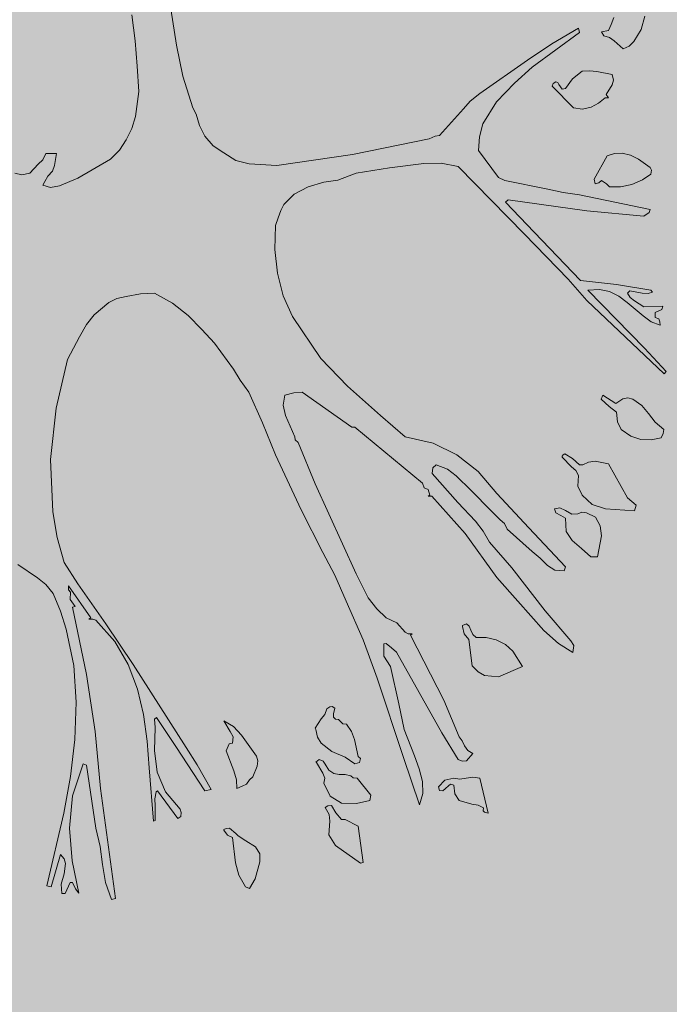
# Model space of a CAD drawing. Units: inches. Extents: x 84 to 1044, y -280 to 906.
# Tile 76 of 105: x 720.2 to 732.52, y 481.17 to 499.87. Entities that reach past the tile are written whole.
import ezdxf

# ---------------------------------------------------------------- set-up
doc = ezdxf.new("R2010")
doc.units = ezdxf.units.IN
doc.layers.add('A-ANNO-DIMS', color=2, linetype='Continuous', lineweight=18)
doc.layers.add('L-PLNT', color=114, linetype='Continuous', lineweight=15)
doc.layers.add('L-PLNT-PATT', color=9, linetype='Continuous', lineweight=9, true_color=0xafd9aa)
doc.styles.get("Standard").update_dxf_attribs({"font": 'arial.ttf'})
doc.dimstyles.get("Standard").update_dxf_attribs({"dimtxt": 0.18, "dimasz": 0.18, "dimexe": 0.18, "dimexo": 0.0625, "dimgap": 0.09, "dimtad": 0, "dimtih": 1, "dimtoh": 1, "dimdec": 4, "dimzin": 0, "dimdsep": 46, "dimtxsty": 'Standard', "dimcen": 0.09, "dimadec": 0, "dimazin": 0, "dimtfac": 1, "dimtdec": 4, "dimtofl": 0, "dimtmove": 0, "dimatfit": 3, "dimfxl": 1, "dimtolj": 1, "dimtzin": 0, "dimarcsym": 0})

# ---------------------------------------------------------------- blocks, each defined once
blk = doc.blocks.new('A$C37E508DF')
for p, q in [((0.7911, 1.1436), (0.8027, 1.0677)), ((0.7512, 1.0728), (0.7469, 1.1054)), ((1.3455, 1.0934), (1.3485, 1.102)), ((1.3875, 1.1037), (1.3828, 1.087)), ((1.3057, 1.0835), (1.2469, 1.0402)), ((1.2713, 1.0694), (1.3044, 1.0887)), ((1.3044, 1.0887), (1.3057, 1.0835)), ((1.3335, 1.0844), (1.3421, 1.0861)), ((1.3361, 1.0793), (1.3335, 1.0844)), ((1.3421, 1.0861), (1.3455, 1.0934)), ((1.3828, 1.087), (1.3738, 1.072)), ((0.7538, 1.0415), (0.7512, 1.0728)), ((1.3434, 1.0771), (1.3361, 1.0793)), ((1.349, 1.0728), (1.3434, 1.0771)), ((1.3605, 1.063), (1.349, 1.0728)), ((1.3738, 1.072), (1.3678, 1.0664)), ((0.8027, 1.0677), (0.8108, 1.0287)), ((1.2409, 1.0488), (1.2713, 1.0694)), ((1.3678, 1.0664), (1.3605, 1.063)), ((1.1813, 1.0072), (1.2409, 1.0488)), ((0.7559, 1.0098), (0.7538, 1.0415)), ((1.2469, 1.0402), (1.2246, 1.0201)), ((1.2971, 1.0257), (1.3091, 1.0351)), ((1.3091, 1.0351), (1.3185, 1.0355)), ((1.3185, 1.0355), (1.3275, 1.0347)), ((1.3275, 1.0347), (1.3468, 1.0308)), ((0.8108, 1.0287), (0.8233, 0.9892)), ((1.2731, 1.0197), (1.2761, 1.0218)), ((1.2761, 1.0218), (1.2786, 1.0209)), ((1.2885, 1.0136), (1.2971, 1.0257)), ((1.3468, 1.0308), (1.3481, 1.0239)), ((1.3481, 1.0239), (1.3468, 1.018)), ((0.7516, 0.9785), (0.7559, 1.0098)), ((1.2246, 1.0201), (1.2023, 0.9969)), ((1.2718, 1.0162), (1.2731, 1.0197)), ((1.2984, 0.9892), (1.2718, 1.0162)), ((1.2786, 1.0209), (1.2799, 1.0184)), ((1.2799, 1.0184), (1.2842, 1.0124)), ((1.2842, 1.0124), (1.2885, 1.0136)), ((1.3468, 1.018), (1.3391, 1.0059)), ((1.1612, 0.9879), (1.1693, 0.9974)), ((1.1693, 0.9974), (1.1813, 1.0072)), ((1.2023, 0.9969), (1.1852, 0.9691)), ((1.3378, 1.0016), (1.3297, 0.9952)), ((1.3421, 1.0016), (1.3378, 1.0016)), ((1.3391, 1.0059), (1.3421, 1.0016)), ((0.8233, 0.9892), (0.8275, 0.9815)), ((1.1311, 0.9549), (1.1612, 0.9879)), ((1.3095, 0.9875), (1.2984, 0.9892)), ((1.3202, 0.9901), (1.3095, 0.9875)), ((1.3297, 0.9952), (1.3202, 0.9901)), ((0.7469, 0.9635), (0.7516, 0.9785)), ((0.8275, 0.9815), (0.8314, 0.9673)), ((0.7401, 0.9493), (0.7469, 0.9635)), ((0.8314, 0.9673), (0.8383, 0.954)), ((1.1852, 0.9691), (1.1809, 0.9532)), ((0.7315, 0.9365), (0.7401, 0.9493)), ((0.8383, 0.954), (0.8486, 0.942)), ((1.0227, 0.9309), (1.1183, 0.9506)), ((1.1183, 0.9506), (1.1256, 0.954)), ((1.1256, 0.954), (1.1311, 0.9549)), ((1.1809, 0.9532), (1.1796, 0.936)), ((0.7203, 0.9253), (0.7315, 0.9365)), ((0.8486, 0.942), (0.8619, 0.933)), ((1.1796, 0.936), (1.2049, 0.9022)), ((0.6303, 0.9189), (0.6359, 0.9245)), ((0.6359, 0.9245), (0.6397, 0.9322)), ((0.6397, 0.9322), (0.653, 0.9322)), ((0.653, 0.9322), (0.6505, 0.9172)), ((0.6796, 0.9013), (0.7203, 0.9253)), ((0.8619, 0.933), (0.8769, 0.9236)), ((0.8769, 0.9236), (0.8936, 0.9193)), ((0.9279, 0.9172), (1.0227, 0.9309)), ((1.3241, 0.9), (1.3404, 0.9292)), ((1.3404, 0.9292), (1.3494, 0.9322)), ((1.3494, 0.9322), (1.3592, 0.9326)), ((1.3592, 0.9326), (1.3695, 0.93)), ((1.3695, 0.93), (1.3794, 0.9253)), ((1.3794, 0.9253), (1.394, 0.9146)), ((0.6196, 0.9077), (0.6303, 0.9189)), ((0.6505, 0.9172), (0.6479, 0.9103)), ((0.8936, 0.9193), (0.9279, 0.9172)), ((1.0685, 0.9142), (1.0269, 0.9077)), ((1.1114, 0.9198), (1.0685, 0.9142)), ((1.1333, 0.9202), (1.1114, 0.9198)), ((1.1543, 0.9159), (1.1333, 0.9202)), ((1.2371, 0.8314), (1.1543, 0.9159)), ((1.394, 0.9146), (1.3957, 0.9112)), ((1.3957, 0.9112), (1.3948, 0.9065)), ((0.6011, 0.9077), (0.6097, 0.9056)), ((0.6097, 0.9056), (0.6196, 0.9077)), ((0.6423, 0.9039), (0.6384, 0.8974)), ((0.6479, 0.9103), (0.6423, 0.9039)), ((0.6569, 0.8919), (0.6796, 0.9013)), ((1.0042, 0.8987), (0.9866, 0.8962)), ((1.0269, 0.9077), (1.0042, 0.8987)), ((1.2049, 0.9022), (1.2126, 0.8983)), ((1.2126, 0.8983), (1.2662, 0.8876)), ((1.3254, 0.8944), (1.3241, 0.9)), ((1.3335, 0.8983), (1.3301, 0.8957)), ((1.3395, 0.8944), (1.3335, 0.8983)), ((1.3846, 0.8992), (1.3713, 0.8936)), ((1.3948, 0.9065), (1.3846, 0.8992)), ((0.6384, 0.8974), (0.6359, 0.8927)), ((0.6359, 0.8927), (0.6457, 0.8897)), ((0.6457, 0.8897), (0.6569, 0.8919)), ((0.9673, 0.8906), (0.9498, 0.8816)), ((0.9866, 0.8962), (0.9673, 0.8906)), ((1.2662, 0.8876), (1.2855, 0.8833)), ((1.3301, 0.8957), (1.3254, 0.8944)), ((1.3434, 0.8906), (1.3395, 0.8944)), ((1.3571, 0.8906), (1.3434, 0.8906)), ((1.3713, 0.8936), (1.3571, 0.8906)), ((0.9498, 0.8816), (0.9369, 0.8687)), ((1.2169, 0.8743), (1.2135, 0.8713)), ((1.3151, 0.8606), (1.2169, 0.8743)), ((1.2855, 0.8833), (1.3057, 0.8807)), ((1.3057, 0.8807), (1.394, 0.8623)), ((0.9369, 0.8687), (0.933, 0.861)), ((1.2135, 0.8713), (1.2491, 0.834)), ((1.394, 0.8623), (1.3927, 0.8584)), ((0.9296, 0.852), (0.9262, 0.8421)), ((0.933, 0.861), (0.9296, 0.852)), ((1.3863, 0.8541), (1.3151, 0.8606)), ((1.3927, 0.8584), (1.3863, 0.8541)), ((0.9262, 0.8421), (0.9257, 0.8121)), ((1.2919, 0.7752), (1.2371, 0.8314)), ((1.2491, 0.834), (1.3069, 0.7735)), ((0.9257, 0.8121), (0.9287, 0.7825)), ((0.9287, 0.7825), (0.936, 0.7542)), ((1.3151, 0.7487), (1.2919, 0.7752)), ((1.3069, 0.7735), (1.352, 0.7684)), ((1.352, 0.7684), (1.3948, 0.7615)), ((0.7285, 0.7512), (0.7182, 0.7461)), ((0.7401, 0.7534), (0.7285, 0.7512)), ((0.7577, 0.7568), (0.7401, 0.7534)), ((0.7752, 0.7577), (0.7577, 0.7568)), ((0.798, 0.7452), (0.7752, 0.7577)), ((0.936, 0.7542), (0.9476, 0.7285)), ((1.3309, 0.7624), (1.3164, 0.7615)), ((1.3164, 0.7615), (1.3871, 0.6891)), ((1.3434, 0.7598), (1.3309, 0.7624)), ((1.355, 0.7538), (1.3434, 0.7598)), ((1.3653, 0.7461), (1.355, 0.7538)), ((1.3687, 0.7607), (1.3657, 0.7577)), ((1.3657, 0.7577), (1.3691, 0.7521)), ((1.3841, 0.7577), (1.3687, 0.7607)), ((1.3691, 0.7521), (1.3743, 0.7482)), ((1.3914, 0.7572), (1.3841, 0.7577)), ((1.397, 0.759), (1.3914, 0.7572)), ((1.3948, 0.7615), (1.397, 0.759)), ((0.7182, 0.7461), (0.7002, 0.7307)), ((0.8173, 0.7298), (0.798, 0.7452)), ((1.3391, 0.7255), (1.3151, 0.7487)), ((1.3854, 0.7294), (1.3653, 0.7461)), ((1.3743, 0.7482), (1.3863, 0.7405)), ((1.3863, 0.7405), (1.4099, 0.7414)), ((1.4099, 0.7414), (1.4086, 0.7375)), ((0.7002, 0.7307), (0.6903, 0.7186)), ((0.8344, 0.7122), (0.8173, 0.7298)), ((0.9476, 0.7285), (0.9828, 0.6762)), ((1.3953, 0.7221), (1.3854, 0.7294)), ((1.4086, 0.7375), (1.4004, 0.7337)), ((1.4004, 0.7337), (1.4004, 0.7272)), ((1.4004, 0.7272), (1.4047, 0.7255)), ((0.6903, 0.7186), (0.6818, 0.7032)), ((1.4116, 0.6569), (1.3391, 0.7255)), ((1.4064, 0.7178), (1.3953, 0.7221)), ((1.4047, 0.7255), (1.406, 0.7221)), ((1.406, 0.7221), (1.4064, 0.7178)), ((0.6818, 0.7032), (0.6667, 0.6749)), ((0.8503, 0.6951), (0.8344, 0.7122)), ((0.8739, 0.6629), (0.8503, 0.6951)), ((1.3871, 0.6891), (1.4141, 0.6599)), ((0.6667, 0.6749), (0.6526, 0.614)), ((0.9828, 0.6762), (1.0162, 0.6415)), ((0.8824, 0.6492), (0.8739, 0.6629)), ((1.4141, 0.6599), (1.4116, 0.6569)), ((0.8932, 0.6342), (0.8824, 0.6492)), ((1.0162, 0.6415), (1.0574, 0.605)), ((0.9103, 0.5956), (0.8932, 0.6342)), ((0.9382, 0.6303), (0.936, 0.6179)), ((0.9493, 0.6333), (0.9382, 0.6303)), ((0.9596, 0.6342), (0.9493, 0.6333)), ((1.0218, 0.5904), (0.9596, 0.6342)), ((1.3327, 0.6252), (1.3348, 0.6303)), ((1.3348, 0.6303), (1.3511, 0.62)), ((0.936, 0.6179), (0.939, 0.605)), ((1.343, 0.6162), (1.3327, 0.6252)), ((1.352, 0.6089), (1.343, 0.6162)), ((1.3511, 0.62), (1.3601, 0.6256)), ((1.3601, 0.6256), (1.3661, 0.6269)), ((1.3661, 0.6269), (1.3725, 0.6252)), ((1.3725, 0.6252), (1.3837, 0.6175)), ((1.3837, 0.6175), (1.3918, 0.6072)), ((0.6526, 0.614), (0.6457, 0.5497)), ((0.939, 0.605), (0.9506, 0.5784)), ((1.0574, 0.605), (1.0883, 0.5784)), ((1.3533, 0.5969), (1.352, 0.6089)), ((1.3918, 0.6072), (1.4004, 0.5964)), ((0.9262, 0.5557), (0.9103, 0.5956)), ((1.358, 0.5874), (1.3533, 0.5969)), ((1.4004, 0.5964), (1.4111, 0.5874)), ((0.9506, 0.5784), (0.951, 0.5746)), ((1.0256, 0.5904), (1.0218, 0.5904)), ((1.1097, 0.5205), (1.0256, 0.5904)), ((1.0883, 0.5784), (1.123, 0.5703)), ((1.37, 0.5789), (1.358, 0.5874)), ((1.3824, 0.575), (1.37, 0.5789)), ((1.4103, 0.5823), (1.4077, 0.5771)), ((1.4111, 0.5874), (1.4103, 0.5823)), ((0.951, 0.5746), (0.9545, 0.5711)), ((0.9545, 0.5711), (0.9759, 0.5193)), ((1.123, 0.5703), (1.1526, 0.5557)), ((1.3953, 0.5746), (1.3824, 0.575)), ((1.4077, 0.5771), (1.3953, 0.5746)), ((0.9583, 0.4871), (0.9262, 0.5557)), ((1.1526, 0.5557), (1.1792, 0.5347)), ((1.2842, 0.554), (1.2855, 0.5557)), ((1.2842, 0.5527), (1.2842, 0.554)), ((1.2855, 0.5557), (1.2876, 0.557)), ((1.2876, 0.557), (1.2971, 0.551)), ((0.6457, 0.5497), (0.6483, 0.4845)), ((1.1268, 0.5433), (1.1226, 0.5394)), ((1.141, 0.5377), (1.1268, 0.5433)), ((1.2958, 0.5407), (1.2842, 0.5527)), ((1.2971, 0.551), (1.3057, 0.5433)), ((1.3057, 0.5433), (1.3099, 0.5433)), ((1.3099, 0.5433), (1.3172, 0.5467)), ((1.3172, 0.5467), (1.3254, 0.548)), ((1.3254, 0.548), (1.3421, 0.5446)), ((1.3421, 0.5446), (1.3657, 0.5021)), ((1.1226, 0.5394), (1.1221, 0.5325)), ((1.1221, 0.5325), (1.1539, 0.4961)), ((1.1521, 0.5296), (1.141, 0.5377)), ((1.1706, 0.5111), (1.1521, 0.5296)), ((1.1792, 0.5347), (1.2027, 0.5072)), ((1.3014, 0.536), (1.2958, 0.5407)), ((1.3044, 0.53), (1.3014, 0.536)), ((1.3039, 0.5167), (1.3044, 0.53)), ((0.9759, 0.5193), (1.0269, 0.4069)), ((1.1118, 0.5145), (1.1097, 0.5205)), ((1.117, 0.5124), (1.1118, 0.5145)), ((1.1191, 0.5055), (1.117, 0.5124)), ((1.117, 0.5042), (1.1191, 0.5055)), ((1.1955, 0.4858), (1.1706, 0.5111)), ((1.2027, 0.5072), (1.2426, 0.4644)), ((1.3091, 0.5055), (1.3039, 0.5167)), ((1.3215, 0.4935), (1.3091, 0.5055)), ((1.1217, 0.5042), (1.117, 0.5042)), ((1.1633, 0.4575), (1.1217, 0.5042)), ((1.1539, 0.4961), (1.1762, 0.4729)), ((1.3382, 0.4884), (1.3215, 0.4935)), ((1.3657, 0.5021), (1.3764, 0.4927)), ((1.3764, 0.4927), (1.3743, 0.4858)), ((0.6483, 0.4845), (0.6539, 0.4524)), ((0.9853, 0.4335), (0.9583, 0.4871)), ((1.207, 0.4747), (1.1955, 0.4858)), ((1.2748, 0.4884), (1.2812, 0.4897)), ((1.2761, 0.4832), (1.2748, 0.4884)), ((1.2825, 0.4798), (1.2761, 0.4832)), ((1.2812, 0.4897), (1.2885, 0.4862)), ((1.2885, 0.4764), (1.2825, 0.4798)), ((1.2885, 0.4862), (1.2962, 0.4815)), ((1.2962, 0.4815), (1.3039, 0.482)), ((1.3039, 0.482), (1.3087, 0.4841)), ((1.3087, 0.4841), (1.3147, 0.4832)), ((1.3147, 0.4832), (1.3258, 0.4777)), ((1.3743, 0.4858), (1.3382, 0.4884)), ((1.1762, 0.4729), (1.1856, 0.4605)), ((1.2122, 0.47), (1.207, 0.4747)), ((1.2156, 0.4627), (1.2122, 0.47)), ((1.2894, 0.4601), (1.2885, 0.4764)), ((1.3258, 0.4777), (1.3318, 0.4669)), ((1.2027, 0.4026), (1.1633, 0.4575)), ((1.1856, 0.4605), (1.1933, 0.4468)), ((1.2469, 0.4348), (1.2156, 0.4627)), ((1.2426, 0.4644), (1.2885, 0.4159)), ((1.2967, 0.4485), (1.2894, 0.4601)), ((1.3318, 0.4669), (1.3331, 0.4545)), ((0.6539, 0.4524), (0.6625, 0.4211)), ((1.1933, 0.4468), (1.2212, 0.4146)), ((1.3082, 0.4386), (1.2967, 0.4485)), ((1.3331, 0.4545), (1.3284, 0.4284)), ((1.0003, 0.4052), (0.9853, 0.4335)), ((1.2568, 0.4266), (1.2469, 0.4348)), ((1.3198, 0.4284), (1.3082, 0.4386)), ((0.6295, 0.4022), (0.6046, 0.4189)), ((0.6625, 0.4211), (0.6796, 0.3945)), ((1.2658, 0.4176), (1.2568, 0.4266)), ((1.3284, 0.4284), (1.3198, 0.4284)), ((1.0269, 0.4069), (1.0419, 0.3769)), ((1.2212, 0.4146), (1.2628, 0.361)), ((1.2752, 0.4116), (1.2658, 0.4176)), ((1.2868, 0.4108), (1.2752, 0.4116)), ((1.2885, 0.4159), (1.2868, 0.4108)), ((0.6397, 0.3936), (0.6295, 0.4022)), ((0.6796, 0.3945), (0.7148, 0.3447)), ((1.0145, 0.373), (1.0003, 0.4052)), ((1.2289, 0.373), (1.2027, 0.4026)), ((0.6487, 0.3825), (0.6397, 0.3936)), ((0.6582, 0.3602), (0.6487, 0.3825)), ((0.6959, 0.352), (0.668, 0.3919)), ((0.668, 0.3919), (0.668, 0.3872)), ((0.668, 0.3872), (0.6706, 0.3842)), ((0.6706, 0.3842), (0.6702, 0.3748)), ((0.6702, 0.3748), (0.6762, 0.3662)), ((1.0359, 0.3246), (1.0145, 0.373)), ((1.0419, 0.3769), (1.0527, 0.3632)), ((1.2615, 0.3362), (1.2289, 0.373)), ((0.665, 0.3379), (0.6582, 0.3602)), ((0.6762, 0.3662), (0.6732, 0.3653)), ((0.6732, 0.3653), (0.6903, 0.2813)), ((1.0527, 0.3632), (1.0647, 0.352)), ((1.2628, 0.361), (1.2949, 0.3233)), ((0.6933, 0.3503), (0.6959, 0.352)), ((0.6985, 0.3503), (0.6933, 0.3503)), ((0.7023, 0.349), (0.6985, 0.3503)), ((0.7259, 0.3224), (0.7023, 0.349)), ((0.7148, 0.3447), (0.7487, 0.2937)), ((1.0647, 0.352), (1.078, 0.346)), ((1.078, 0.346), (1.0883, 0.334)), ((1.1599, 0.3426), (1.1646, 0.3447)), ((1.1646, 0.3447), (1.168, 0.3417)), ((0.6745, 0.2924), (0.665, 0.3379)), ((1.0883, 0.334), (1.0921, 0.3319)), ((1.1599, 0.3413), (1.1599, 0.3426)), ((1.162, 0.3319), (1.1599, 0.3413)), ((1.168, 0.3417), (1.1702, 0.3366)), ((1.1702, 0.3366), (1.1727, 0.3314)), ((1.2795, 0.3199), (1.2615, 0.3362)), ((0.7427, 0.2937), (0.7259, 0.3224)), ((1.0535, 0.2766), (1.0359, 0.3246)), ((1.0647, 0.3199), (1.0617, 0.3194)), ((1.0711, 0.3147), (1.0647, 0.3199)), ((1.0921, 0.3319), (1.0968, 0.3319)), ((1.0968, 0.3319), (1.0947, 0.3306)), ((1.0947, 0.3306), (1.1367, 0.2491)), ((1.1676, 0.325), (1.162, 0.3319)), ((1.1719, 0.292), (1.1676, 0.325)), ((1.1727, 0.3314), (1.177, 0.3276)), ((1.177, 0.3276), (1.1895, 0.3276)), ((1.1895, 0.3276), (1.2019, 0.3246)), ((1.2019, 0.3246), (1.2135, 0.3186)), ((1.2975, 0.3087), (1.2795, 0.3199)), ((1.2949, 0.3233), (1.2988, 0.3173)), ((1.0617, 0.3194), (1.0617, 0.304)), ((1.0775, 0.3092), (1.0711, 0.3147)), ((1.1341, 0.2084), (1.0775, 0.3092)), ((1.2135, 0.3186), (1.2225, 0.3104)), ((1.2225, 0.3104), (1.2349, 0.2911)), ((1.2988, 0.3173), (1.2975, 0.3087)), ((1.0617, 0.304), (1.0698, 0.2911)), ((0.6775, 0.2465), (0.6745, 0.2924)), ((0.7542, 0.2628), (0.7427, 0.2937)), ((0.7487, 0.2937), (0.8151, 0.1899)), ((1.0698, 0.2911), (1.0805, 0.2448)), ((1.1792, 0.2847), (1.1719, 0.292)), ((1.1873, 0.28), (1.1792, 0.2847)), ((1.2349, 0.2911), (1.2049, 0.2783)), ((0.6903, 0.2813), (0.7015, 0.2101)), ((1.0861, 0.1775), (1.0535, 0.2766)), ((1.2049, 0.2783), (1.1873, 0.28)), ((0.7615, 0.2311), (0.7542, 0.2628)), ((0.6758, 0.2002), (0.6775, 0.2465)), ((1.1367, 0.2491), (1.1556, 0.2032)), ((0.9879, 0.2311), (0.9905, 0.2384)), ((0.9905, 0.2384), (0.9943, 0.241)), ((0.9943, 0.241), (0.9973, 0.2414)), ((0.9973, 0.2414), (1.0003, 0.2393)), ((1.0003, 0.2393), (0.9986, 0.232)), ((1.0805, 0.2448), (1.087, 0.2127)), ((0.7662, 0.1981), (0.7615, 0.2311)), ((0.7778, 0.2277), (0.7752, 0.2255)), ((0.7752, 0.2255), (0.7761, 0.2152)), ((0.8018, 0.1912), (0.7778, 0.2277)), ((0.8619, 0.2234), (0.8739, 0.2161)), ((0.87, 0.2101), (0.8619, 0.2234)), ((0.9759, 0.214), (0.9836, 0.226)), ((0.9836, 0.226), (0.9879, 0.2311)), ((0.9986, 0.232), (0.9986, 0.2281)), ((0.9986, 0.2281), (1.0012, 0.2255)), ((1.0012, 0.2255), (1.0051, 0.2251)), ((1.0051, 0.2251), (1.0076, 0.2225)), ((1.0076, 0.2225), (1.0106, 0.2195)), ((0.7015, 0.2101), (0.7079, 0.1389)), ((0.7761, 0.2152), (0.7752, 0.1861)), ((0.8734, 0.2032), (0.87, 0.2101)), ((0.8739, 0.2161), (0.8841, 0.2054)), ((0.9768, 0.2127), (0.9759, 0.214)), ((0.9789, 0.2028), (0.9768, 0.2127)), ((1.0106, 0.2195), (1.0149, 0.2191)), ((1.0149, 0.2191), (1.0214, 0.2101)), ((1.0214, 0.2101), (1.0252, 0.2002)), ((1.087, 0.2127), (1.0998, 0.1797)), ((0.6706, 0.1539), (0.6758, 0.2002)), ((0.7688, 0.1646), (0.7662, 0.1981)), ((0.8726, 0.1955), (0.8734, 0.2032)), ((0.8841, 0.2054), (0.9026, 0.1792)), ((0.9832, 0.1955), (0.9789, 0.2028)), ((1.0252, 0.2002), (1.0295, 0.1788)), ((1.1543, 0.1749), (1.1341, 0.2084)), ((1.1556, 0.2032), (1.1594, 0.1985)), ((1.1594, 0.1985), (1.1624, 0.1921)), ((0.7752, 0.1861), (0.7787, 0.1591)), ((0.8383, 0.1359), (0.8018, 0.1912)), ((0.8151, 0.1899), (0.8288, 0.1685)), ((0.8649, 0.1857), (0.8687, 0.1947)), ((0.8743, 0.1608), (0.8649, 0.1857)), ((0.8687, 0.1947), (0.8726, 0.1955)), ((0.9969, 0.1852), (0.9832, 0.1955)), ((1.0132, 0.1779), (0.9969, 0.1852)), ((1.1624, 0.1921), (1.1663, 0.1861)), ((1.1663, 0.1861), (1.1727, 0.1827)), ((0.9026, 0.1792), (0.9043, 0.1732)), ((0.9043, 0.1732), (0.9035, 0.1668)), ((0.9768, 0.1719), (0.9811, 0.1749)), ((0.9811, 0.1749), (0.9858, 0.1728)), ((0.9858, 0.1728), (0.9884, 0.1694)), ((1.0256, 0.1698), (1.0132, 0.1779)), ((1.0295, 0.1788), (1.0325, 0.1762)), ((1.0325, 0.1762), (1.0312, 0.1711)), ((1.1063, 0.1183), (1.0861, 0.1775)), ((1.0998, 0.1797), (1.1058, 0.1634)), ((1.1594, 0.1728), (1.1543, 0.1749)), ((1.1646, 0.1732), (1.1594, 0.1728)), ((1.1727, 0.1827), (1.1646, 0.1732)), ((0.6865, 0.1698), (0.6732, 0.1295)), ((0.6903, 0.1681), (0.6865, 0.1698)), ((0.7023, 0.0892), (0.6903, 0.1681)), ((0.774, 0.0982), (0.7688, 0.1646)), ((0.8288, 0.1685), (0.846, 0.1376)), ((0.8777, 0.1496), (0.8743, 0.1608)), ((0.9035, 0.1668), (0.8983, 0.1535)), ((0.9776, 0.1711), (0.9768, 0.1719)), ((0.9853, 0.1578), (0.9776, 0.1711)), ((0.9884, 0.1694), (0.9931, 0.1616)), ((0.9931, 0.1616), (0.9991, 0.1574)), ((1.0312, 0.1711), (1.0256, 0.1698)), ((1.1058, 0.1634), (1.1097, 0.1475)), ((0.662, 0.108), (0.6706, 0.1539)), ((0.7787, 0.1591), (0.789, 0.1346)), ((0.8781, 0.1389), (0.8777, 0.1496)), ((0.894, 0.1496), (0.8902, 0.1441)), ((0.8983, 0.1535), (0.894, 0.1496)), ((0.9879, 0.1518), (0.9853, 0.1578)), ((0.9866, 0.1453), (0.9879, 0.1518)), ((0.9991, 0.1574), (1.0059, 0.1565)), ((1.0059, 0.1565), (1.0132, 0.1565)), ((1.0132, 0.1565), (1.0205, 0.1548)), ((1.0205, 0.1548), (1.0235, 0.1522)), ((1.0235, 0.1522), (1.0282, 0.1518)), ((1.0282, 0.1518), (1.0454, 0.1303)), ((1.1298, 0.1411), (1.1376, 0.1492)), ((1.1376, 0.1492), (1.1491, 0.1518)), ((1.1491, 0.1518), (1.1564, 0.1505)), ((1.1564, 0.1505), (1.1642, 0.1518)), ((1.1642, 0.1518), (1.1727, 0.1531)), ((1.1727, 0.1531), (1.1813, 0.1518)), ((1.1813, 0.1518), (1.192, 0.108)), ((0.7079, 0.1389), (0.7268, 0.0013)), ((0.7791, 0.1359), (0.7774, 0.1346)), ((0.8044, 0.1012), (0.7791, 0.1359)), ((0.846, 0.1376), (0.8383, 0.1359)), ((0.8846, 0.1419), (0.8781, 0.1389)), ((0.8902, 0.1441), (0.8846, 0.1419)), ((0.9948, 0.1291), (0.9866, 0.1453)), ((1.1097, 0.1475), (1.1101, 0.1325)), ((1.1311, 0.1364), (1.1298, 0.1411)), ((1.1354, 0.1359), (1.1311, 0.1364)), ((1.1384, 0.1389), (1.1354, 0.1359)), ((1.1423, 0.1423), (1.1384, 0.1389)), ((1.1449, 0.1441), (1.1423, 0.1423)), ((1.1491, 0.1428), (1.1449, 0.1441)), ((1.1504, 0.132), (1.1491, 0.1428)), ((0.6732, 0.1295), (0.6693, 0.0892)), ((0.7774, 0.1346), (0.7757, 0.1261)), ((0.7757, 0.1261), (0.7761, 0.117)), ((0.789, 0.1346), (0.8074, 0.1132)), ((1.0089, 0.1205), (0.9948, 0.1291)), ((1.0441, 0.1239), (1.0274, 0.12)), ((1.0454, 0.1303), (1.0441, 0.1239)), ((1.1101, 0.1325), (1.1063, 0.1183)), ((1.1556, 0.1239), (1.1504, 0.132)), ((1.1714, 0.1192), (1.1556, 0.1239)), ((0.7761, 0.117), (0.7761, 0.099)), ((0.8074, 0.1132), (0.8087, 0.1089)), ((0.9884, 0.1149), (0.9918, 0.117)), ((0.9935, 0.1063), (0.9884, 0.1149)), ((0.9918, 0.117), (0.9961, 0.1175)), ((0.9961, 0.1175), (1.0016, 0.1085)), ((1.0274, 0.12), (1.0089, 0.1205)), ((1.1792, 0.1179), (1.1714, 0.1192)), ((1.186, 0.1145), (1.1792, 0.1179)), ((1.1856, 0.111), (1.186, 0.1145)), ((1.1873, 0.1093), (1.1856, 0.111)), ((0.641, 0.0172), (0.662, 0.108)), ((0.7761, 0.099), (0.774, 0.0982)), ((0.8083, 0.1037), (0.8044, 0.1012)), ((0.8087, 0.1089), (0.8083, 0.1037)), ((0.9943, 0.0982), (0.9935, 0.1063)), ((1.0016, 0.1085), (1.0089, 0.0999)), ((1.0089, 0.0999), (1.0132, 0.0999)), ((1.0132, 0.0999), (1.0295, 0.0917)), ((1.192, 0.108), (1.1873, 0.1093)), ((0.6693, 0.0892), (0.6728, 0.0484)), ((0.7075, 0.0665), (0.7023, 0.0892)), ((0.8619, 0.0875), (0.8649, 0.0887)), ((0.8619, 0.0866), (0.8619, 0.0875)), ((0.8666, 0.0806), (0.8619, 0.0866)), ((0.8649, 0.0887), (0.8691, 0.0892)), ((0.8691, 0.0892), (0.8769, 0.0827)), ((0.9931, 0.081), (0.9943, 0.0982)), ((1.0295, 0.0917), (1.0359, 0.0463)), ((0.8726, 0.0776), (0.8666, 0.0806)), ((0.8764, 0.0459), (0.8726, 0.0776)), ((0.8769, 0.0827), (0.8799, 0.0797)), ((0.8799, 0.0797), (0.8893, 0.0733)), ((1.0012, 0.0677), (0.9931, 0.081)), ((0.7105, 0.0437), (0.7075, 0.0665)), ((0.8893, 0.0733), (0.9013, 0.066)), ((0.9013, 0.066), (0.9069, 0.057)), ((1.0325, 0.0454), (1.0012, 0.0677)), ((0.6582, 0.0562), (0.6466, 0.0159)), ((0.6625, 0.051), (0.6582, 0.0562)), ((0.6642, 0.045), (0.6625, 0.051)), ((0.9069, 0.057), (0.9069, 0.0471)), ((0.6625, 0.0321), (0.6642, 0.045)), ((0.6728, 0.0484), (0.6809, 0.0082)), ((0.7144, 0.0214), (0.7105, 0.0437)), ((0.8807, 0.0304), (0.8764, 0.0459)), ((0.9069, 0.0471), (0.9009, 0.0261)), ((1.0359, 0.0463), (1.0325, 0.0454)), ((0.659, 0.0193), (0.6625, 0.0321)), ((0.8889, 0.0159), (0.8807, 0.0304)), ((0.9009, 0.0261), (0.894, 0.0137)), ((0.6466, 0.0159), (0.641, 0.0172)), ((0.6595, 0.0077), (0.659, 0.0193)), ((0.6702, 0.0214), (0.6637, 0.0077)), ((0.6732, 0.0214), (0.6702, 0.0214)), ((0.6766, 0.0133), (0.6732, 0.0214)), ((0.6809, 0.0082), (0.6766, 0.0133)), ((0.7216, 0), (0.7144, 0.0214)), ((0.894, 0.0137), (0.8889, 0.0159)), ((0.6637, 0.0077), (0.6595, 0.0077)), ((0.7268, 0.0013), (0.7216, 0))]:
    blk.add_line(p, q)
blk = doc.blocks.new('*D62')
at = {"layer": 'A-ANNO-DIMS', "color": 0, "lineweight": -2, "transparency": 16777216}
for p, q in [((203.179, 709.183), (203.179, 905.9)), ((896.074, 400.183), (896.074, 905.9)), ((203.359, 905.72), (549.232, 905.72)), ((895.894, 905.72), (550.021, 905.72))]:
    blk.add_line(p, q, dxfattribs=at)
at = {"layer": 'A-ANNO-DIMS', "color": 0, "transparency": 16777216}
for points in [[(203.359, 905.75), (203.359, 905.69), (203.179, 905.72)], [(895.894, 905.75), (895.894, 905.69), (896.074, 905.72)]]:
    blk.add_solid(points, dxfattribs=at)
at = {"layer": 'Defpoints', "color": 0, "transparency": 16777216}
for p in [(896.074, 905.72), (203.179, 709.12), (896.074, 400.12)]:
    blk.add_point(p, dxfattribs=at)
at = {"layer": 'A-ANNO-DIMS', "color": 0, "transparency": 16777216, "insert": (549.627, 905.72), "char_height": 0.18, "attachment_point": 5}
blk.add_mtext('\\A1;692.9', dxfattribs=at)

msp = doc.modelspace()

# ---------------------------------------------------------------- hatches: boundary and pattern name
at = {"layer": 'L-PLNT-PATT', "transparency": 33554597}
h = msp.add_hatch(color=256, dxfattribs=at)
h.dxf.hatch_style = 1
h.paths.add_polyline_path([(896.074, 511.12), (704.074, 511.12), (704.074, 491.62), (704.074, 419.62), (704.074, 400.12), (833.074, 400.12), (896.074, 400.12)])

# ---------------------------------------------------------------- block references
at = {"layer": 'L-PLNT', "xscale": 15.19586232982809, "yscale": 15.19586232982809, "zscale": 15.19586232982809}
msp.add_blockref('A$C37E508DF', (710.97, 483.159), dxfattribs=at)

# ---------------------------------------------------------------- dimensions: what is measured, and where the dimension line sits
at = {"layer": 'A-ANNO-DIMS'}
dim = msp.add_linear_dim(base=(896.074, 905.72), p1=(203.179, 709.12), p2=(896.074, 400.12), dimstyle='Standard', override={"dimdec": 1, "dimlfac": 1, "dimrnd": 0, "dimzin": 0, "dimdsep": 46, "dimlunit": 2}, dxfattribs=at)
dim.commit()
dim.dimension.update_dxf_attribs({"geometry": '*D62', "text_midpoint": (549.627, 905.72)})

doc.saveas('drawing.dxf')
